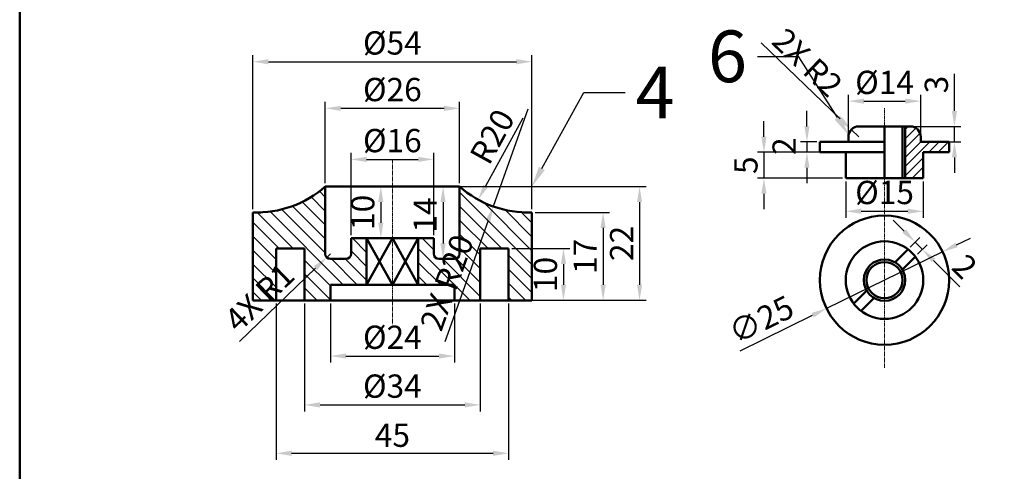
# Model space of a CAD drawing. Units: millimetres. Extents: x 418 to 773, y -46 to 294.
# Tile 4 of 7: x 418 to 609, y 77 to 164. Entities that reach past the tile are written whole.
import ezdxf
from ezdxf import colors
from ezdxf.entities.mleader import LeaderData, LeaderLine
from ezdxf.math import Vec2, Vec3

# ---------------------------------------------------------------- set-up
doc = ezdxf.new("R2010")
doc.units = ezdxf.units.MM
doc.header["$LTSCALE"] = 0.2
doc.linetypes.add('CENTER2', pattern=[28.575, 19.05, -3.175, 3.175, -3.175])
for name, color, linetype, lineweight in [('M-CNTR', 1, 'CENTER2', 18), ('M-DIMS', 2, 'Continuous', 25), ('M-HATC', 8, 'Continuous', 18), ('M-OUTL', 7, 'Continuous', 50), ('M-TEXT', 3, 'Continuous', 25), ('M-TTLB', 7, 'Continuous', 50)]:
    doc.layers.add(name, color=color, linetype=linetype, lineweight=lineweight)
doc.styles.get("Standard").update_dxf_attribs({"font": 'arial.ttf'})
doc.dimstyles.new('ISO-25', dxfattribs={"dimtxt": 4.5, "dimasz": 3, "dimexe": 1.25, "dimexo": 0.625, "dimtad": 1, "dimdec": 1, "dimtxsty": 'Standard', "dimcen": 2.5, "dimadec": 0, "dimazin": 0, "dimtfac": 1, "dimtdec": 1, "dimtmove": 0, "dimatfit": 3, "dimfxl": 1, "dimarcsym": 0})

# ---------------------------------------------------------------- blocks, each defined once
blk = doc.blocks.new('*D22')
at = {"layer": 'Defpoints', "color": 0, "ltscale": 0.2, "transparency": 16777216}
for p in [(517.09, 155.7), (463.09, 126.57), (517.09, 126.57)]:
    blk.add_point(p, dxfattribs=at)
at = {"layer": 'M-DIMS', "color": 0, "lineweight": -2, "ltscale": 0.2, "transparency": 16777216}
for p, q in [((463.09, 127.19), (463.09, 156.95)), ((517.09, 127.19), (517.09, 156.95)), ((466.09, 155.7), (514.09, 155.7))]:
    blk.add_line(p, q, dxfattribs=at)
at = {"layer": 'M-DIMS', "color": 0, "ltscale": 0.2, "transparency": 16777216}
for points in [[(466.09, 156.2), (466.09, 155.2), (463.09, 155.7)], [(514.09, 156.2), (514.09, 155.2), (517.09, 155.7)]]:
    blk.add_solid(points, dxfattribs=at)
at = {"layer": 'M-DIMS', "color": 0, "ltscale": 0.2, "transparency": 16777216, "insert": (490.09, 158.75), "char_height": 4.5, "attachment_point": 5}
blk.add_mtext('%%C54', dxfattribs=at)
blk = doc.blocks.new('*D23')
at = {"layer": 'Defpoints', "color": 0, "ltscale": 0.2, "transparency": 16777216}
for p in [(503.09, 146.69), (477.09, 131.57), (503.09, 131.57)]:
    blk.add_point(p, dxfattribs=at)
at = {"layer": 'M-DIMS', "color": 0, "lineweight": -2, "ltscale": 0.2, "transparency": 16777216}
for p, q in [((477.09, 132.19), (477.09, 147.94)), ((503.09, 132.19), (503.09, 147.94)), ((480.09, 146.69), (500.09, 146.69))]:
    blk.add_line(p, q, dxfattribs=at)
at = {"layer": 'M-DIMS', "color": 0, "ltscale": 0.2, "transparency": 16777216}
for points in [[(480.09, 147.19), (480.09, 146.19), (477.09, 146.69)], [(500.09, 147.19), (500.09, 146.19), (503.09, 146.69)]]:
    blk.add_solid(points, dxfattribs=at)
at = {"layer": 'M-DIMS', "color": 0, "ltscale": 0.2, "transparency": 16777216, "insert": (490.09, 149.74), "char_height": 4.5, "attachment_point": 5}
blk.add_mtext('%%C26', dxfattribs=at)
blk = doc.blocks.new('*D24')
at = {"layer": 'Defpoints', "color": 0, "ltscale": 0.2, "transparency": 16777216}
for p in [(497.65, 131.57), (502.09, 109.57), (537.94, 109.57)]:
    blk.add_point(p, dxfattribs=at)
at = {"layer": 'M-DIMS', "color": 0, "lineweight": -2, "ltscale": 0.2, "transparency": 16777216}
for p, q in [((498.28, 131.57), (539.19, 131.57)), ((537.94, 128.57), (537.94, 112.57)), ((502.72, 109.57), (539.19, 109.57))]:
    blk.add_line(p, q, dxfattribs=at)
at = {"layer": 'M-DIMS', "color": 0, "ltscale": 0.2, "transparency": 16777216}
for points in [[(537.44, 128.57), (538.44, 128.57), (537.94, 131.57)], [(537.44, 112.57), (538.44, 112.57), (537.94, 109.57)]]:
    blk.add_solid(points, dxfattribs=at)
at = {"layer": 'M-DIMS', "color": 0, "ltscale": 0.2, "transparency": 16777216, "insert": (535.05, 120.57), "char_height": 4.5, "attachment_point": 5, "rotation": 90}
blk.add_mtext('22', dxfattribs=at)
blk = doc.blocks.new('*D25')
at = {"layer": 'Defpoints', "color": 0, "ltscale": 0.2, "transparency": 16777216}
for p in [(517.09, 126.57), (517.09, 109.57), (530.88, 109.57)]:
    blk.add_point(p, dxfattribs=at)
at = {"layer": 'M-DIMS', "color": 0, "lineweight": -2, "ltscale": 0.2, "transparency": 16777216}
for p, q in [((517.72, 126.57), (532.13, 126.57)), ((530.88, 123.57), (530.88, 112.57)), ((517.72, 109.57), (532.13, 109.57))]:
    blk.add_line(p, q, dxfattribs=at)
at = {"layer": 'M-DIMS', "color": 0, "ltscale": 0.2, "transparency": 16777216}
for points in [[(530.38, 123.57), (531.38, 123.57), (530.88, 126.57)], [(530.38, 112.57), (531.38, 112.57), (530.88, 109.57)]]:
    blk.add_solid(points, dxfattribs=at)
at = {"layer": 'M-DIMS', "color": 0, "ltscale": 0.2, "transparency": 16777216, "insert": (528, 118.07), "char_height": 4.5, "attachment_point": 5, "rotation": 90}
blk.add_mtext('17', dxfattribs=at)
blk = doc.blocks.new('*D26')
at = {"layer": 'Defpoints', "color": 0, "ltscale": 0.2, "transparency": 16777216}
for p in [(512.59, 119.57), (512.59, 109.57), (523.21, 109.57)]:
    blk.add_point(p, dxfattribs=at)
at = {"layer": 'M-DIMS', "color": 0, "lineweight": -2, "ltscale": 0.2, "transparency": 16777216}
for p, q in [((513.22, 119.57), (524.46, 119.57)), ((523.21, 116.57), (523.21, 112.57)), ((513.22, 109.57), (524.46, 109.57))]:
    blk.add_line(p, q, dxfattribs=at)
at = {"layer": 'M-DIMS', "color": 0, "ltscale": 0.2, "transparency": 16777216}
for points in [[(522.71, 116.57), (523.71, 116.57), (523.21, 119.57)], [(522.71, 112.57), (523.71, 112.57), (523.21, 109.57)]]:
    blk.add_solid(points, dxfattribs=at)
at = {"layer": 'M-DIMS', "color": 0, "ltscale": 0.2, "transparency": 16777216, "insert": (520.29, 114.57), "char_height": 4.5, "attachment_point": 5, "rotation": 90}
blk.add_mtext('10', dxfattribs=at)
blk = doc.blocks.new('*D27')
at = {"layer": 'Defpoints', "color": 0, "ltscale": 0.2, "transparency": 16777216}
for p in [(478.09, 109.57), (502.09, 109.57), (502.09, 98.8)]:
    blk.add_point(p, dxfattribs=at)
at = {"layer": 'M-DIMS', "color": 0, "lineweight": -2, "ltscale": 0.2, "transparency": 16777216}
for p, q in [((478.09, 108.94), (478.09, 97.55)), ((502.09, 108.94), (502.09, 97.55)), ((481.09, 98.8), (499.09, 98.8))]:
    blk.add_line(p, q, dxfattribs=at)
at = {"layer": 'M-DIMS', "color": 0, "ltscale": 0.2, "transparency": 16777216}
for points in [[(481.09, 99.3), (481.09, 98.3), (478.09, 98.8)], [(499.09, 99.3), (499.09, 98.3), (502.09, 98.8)]]:
    blk.add_solid(points, dxfattribs=at)
at = {"layer": 'M-DIMS', "color": 0, "ltscale": 0.2, "transparency": 16777216, "insert": (490.09, 101.85), "char_height": 4.5, "attachment_point": 5}
blk.add_mtext('%%C24', dxfattribs=at)
blk = doc.blocks.new('*D28')
at = {"layer": 'Defpoints', "color": 0, "ltscale": 0.2, "transparency": 16777216}
for p in [(473.09, 109.57), (507.09, 109.57), (507.09, 89.35)]:
    blk.add_point(p, dxfattribs=at)
at = {"layer": 'M-DIMS', "color": 0, "lineweight": -2, "ltscale": 0.2, "transparency": 16777216}
for p, q in [((473.09, 108.94), (473.09, 88.1)), ((507.09, 108.94), (507.09, 88.1)), ((476.09, 89.35), (504.09, 89.35))]:
    blk.add_line(p, q, dxfattribs=at)
at = {"layer": 'M-DIMS', "color": 0, "ltscale": 0.2, "transparency": 16777216}
for points in [[(476.09, 89.85), (476.09, 88.85), (473.09, 89.35)], [(504.09, 89.85), (504.09, 88.85), (507.09, 89.35)]]:
    blk.add_solid(points, dxfattribs=at)
at = {"layer": 'M-DIMS', "color": 0, "ltscale": 0.2, "transparency": 16777216, "insert": (490.09, 92.4), "char_height": 4.5, "attachment_point": 5}
blk.add_mtext('%%C34', dxfattribs=at)
blk = doc.blocks.new('*D29')
at = {"layer": 'Defpoints', "color": 0, "ltscale": 0.2, "transparency": 16777216}
for p in [(467.59, 109.57), (512.59, 109.57), (512.59, 80)]:
    blk.add_point(p, dxfattribs=at)
at = {"layer": 'M-DIMS', "color": 0, "lineweight": -2, "ltscale": 0.2, "transparency": 16777216}
for p, q in [((467.59, 108.94), (467.59, 78.75)), ((512.59, 108.94), (512.59, 78.75)), ((470.59, 80), (509.59, 80))]:
    blk.add_line(p, q, dxfattribs=at)
at = {"layer": 'M-DIMS', "color": 0, "ltscale": 0.2, "transparency": 16777216}
for points in [[(470.59, 80.5), (470.59, 79.5), (467.59, 80)], [(509.59, 80.5), (509.59, 79.5), (512.59, 80)]]:
    blk.add_solid(points, dxfattribs=at)
at = {"layer": 'M-DIMS', "color": 0, "ltscale": 0.2, "transparency": 16777216, "insert": (490.09, 82.91), "char_height": 4.5, "attachment_point": 5}
blk.add_mtext('45', dxfattribs=at)
blk = doc.blocks.new('*D30')
at = {"layer": 'Defpoints', "color": 0, "ltscale": 0.2, "transparency": 16777216}
for p in [(516.34, 146.56), (506.69, 129.03)]:
    blk.add_point(p, dxfattribs=at)
at = {"layer": 'M-DIMS', "color": 0, "lineweight": -2, "ltscale": 0.2, "transparency": 16777216}
blk.add_line((515.37, 144.79), (508.14, 131.66), dxfattribs=at)
at = {"layer": 'M-DIMS', "color": 0, "ltscale": 0.2, "transparency": 16777216}
blk.add_solid([(507.7, 131.9), (508.58, 131.42), (506.69, 129.03)], dxfattribs=at)
at = {"layer": 'M-DIMS', "color": 0, "ltscale": 0.2, "transparency": 16777216, "insert": (509.92, 140.95), "char_height": 4.5, "attachment_point": 5, "rotation": 61.1742}
blk.add_mtext('R20', dxfattribs=at)
blk = doc.blocks.new('*D31')
at = {"layer": 'Defpoints', "color": 0, "ltscale": 0.2, "transparency": 16777216}
for p in [(498.09, 136.82), (482.09, 121.57), (498.09, 121.57)]:
    blk.add_point(p, dxfattribs=at)
at = {"layer": 'M-DIMS', "color": 0, "lineweight": -2, "ltscale": 0.2, "transparency": 16777216}
for p, q in [((482.09, 122.19), (482.09, 138.07)), ((498.09, 122.19), (498.09, 138.07)), ((485.09, 136.82), (495.09, 136.82))]:
    blk.add_line(p, q, dxfattribs=at)
at = {"layer": 'M-DIMS', "color": 0, "ltscale": 0.2, "transparency": 16777216}
for points in [[(485.09, 137.32), (485.09, 136.32), (482.09, 136.82)], [(495.09, 137.32), (495.09, 136.32), (498.09, 136.82)]]:
    blk.add_solid(points, dxfattribs=at)
at = {"layer": 'M-DIMS', "color": 0, "ltscale": 0.2, "transparency": 16777216, "insert": (490.09, 139.87), "char_height": 4.5, "attachment_point": 5}
blk.add_mtext('%%C16', dxfattribs=at)
blk = doc.blocks.new('*D32')
at = {"layer": 'Defpoints', "color": 0, "ltscale": 0.2, "transparency": 16777216}
for p in [(499.92, 131.57), (499.9, 117.57), (500.59, 117.57)]:
    blk.add_point(p, dxfattribs=at)
at = {"layer": 'M-DIMS', "color": 0, "lineweight": -2, "ltscale": 0.2, "transparency": 16777216}
for p, q in [((499.29, 131.57), (498.65, 131.57)), ((499.9, 128.57), (499.9, 120.57)), ((499.97, 117.57), (498.65, 117.57))]:
    blk.add_line(p, q, dxfattribs=at)
at = {"layer": 'M-DIMS', "color": 0, "ltscale": 0.2, "transparency": 16777216}
for points in [[(499.4, 128.57), (500.4, 128.57), (499.9, 131.57)], [(499.4, 120.57), (500.4, 120.57), (499.9, 117.57)]]:
    blk.add_solid(points, dxfattribs=at)
at = {"layer": 'M-DIMS', "color": 0, "ltscale": 0.2, "transparency": 16777216, "insert": (497.02, 126.06), "char_height": 4.5, "attachment_point": 5, "rotation": 90}
blk.add_mtext('14', dxfattribs=at)
blk = doc.blocks.new('*D33')
at = {"layer": 'Defpoints', "color": 0, "ltscale": 0.2, "transparency": 16777216}
for p in [(490.09, 131.57), (487.85, 121.57), (490.09, 121.57)]:
    blk.add_point(p, dxfattribs=at)
at = {"layer": 'M-DIMS', "color": 0, "lineweight": -2, "ltscale": 0.2, "transparency": 16777216}
for p, q in [((489.47, 131.57), (486.6, 131.57)), ((487.85, 128.57), (487.85, 124.57)), ((489.47, 121.57), (486.6, 121.57))]:
    blk.add_line(p, q, dxfattribs=at)
at = {"layer": 'M-DIMS', "color": 0, "ltscale": 0.2, "transparency": 16777216}
for points in [[(487.35, 128.57), (488.35, 128.57), (487.85, 131.57)], [(487.35, 124.57), (488.35, 124.57), (487.85, 121.57)]]:
    blk.add_solid(points, dxfattribs=at)
at = {"layer": 'M-DIMS', "color": 0, "ltscale": 0.2, "transparency": 16777216, "insert": (484.93, 126.57), "char_height": 4.5, "attachment_point": 5, "rotation": 90}
blk.add_mtext('10', dxfattribs=at)
blk = doc.blocks.new('*D34')
at = {"layer": 'Defpoints', "color": 0, "ltscale": 0.2, "transparency": 16777216}
for p in [(592.37, 148.08), (578.37, 141.19), (592.37, 141.19)]:
    blk.add_point(p, dxfattribs=at)
at = {"layer": 'M-DIMS', "color": 0, "lineweight": -2, "ltscale": 0.2, "transparency": 16777216}
for p, q in [((578.37, 141.81), (578.37, 149.33)), ((592.37, 141.81), (592.37, 149.33)), ((581.37, 148.08), (589.37, 148.08))]:
    blk.add_line(p, q, dxfattribs=at)
at = {"layer": 'M-DIMS', "color": 0, "ltscale": 0.2, "transparency": 16777216}
for points in [[(581.37, 148.58), (581.37, 147.58), (578.37, 148.08)], [(589.37, 148.58), (589.37, 147.58), (592.37, 148.08)]]:
    blk.add_solid(points, dxfattribs=at)
at = {"layer": 'M-DIMS', "color": 0, "ltscale": 0.2, "transparency": 16777216, "insert": (585.37, 151.12), "char_height": 4.5, "attachment_point": 5}
blk.add_mtext('%%C14', dxfattribs=at)
blk = doc.blocks.new('*D35')
at = {"layer": 'Defpoints', "color": 0, "ltscale": 0.2, "transparency": 16777216}
for p in [(572.87, 140.19), (570.35, 138.19), (572.87, 138.19)]:
    blk.add_point(p, dxfattribs=at)
at = {"layer": 'M-DIMS', "color": 0, "lineweight": -2, "ltscale": 0.2, "transparency": 16777216}
for p, q in [((570.35, 143.19), (570.35, 146.19)), ((572.24, 140.19), (569.1, 140.19)), ((570.35, 140.19), (570.35, 138.19)), ((572.24, 138.19), (569.1, 138.19)), ((570.35, 135.19), (570.35, 132.19))]:
    blk.add_line(p, q, dxfattribs=at)
at = {"layer": 'M-DIMS', "color": 0, "ltscale": 0.2, "transparency": 16777216}
for points in [[(569.85, 143.19), (570.85, 143.19), (570.35, 140.19)], [(569.85, 135.19), (570.85, 135.19), (570.35, 138.19)]]:
    blk.add_solid(points, dxfattribs=at)
at = {"layer": 'M-DIMS', "color": 0, "ltscale": 0.2, "transparency": 16777216, "insert": (566.51, 139.38), "char_height": 4.5, "attachment_point": 5, "rotation": 90}
blk.add_mtext('2', dxfattribs=at)
blk = doc.blocks.new('*D36')
at = {"layer": 'Defpoints', "color": 0, "ltscale": 0.2, "transparency": 16777216}
for p in [(577.87, 138.19), (562.02, 133.19), (577.87, 133.19)]:
    blk.add_point(p, dxfattribs=at)
at = {"layer": 'M-DIMS', "color": 0, "lineweight": -2, "ltscale": 0.2, "transparency": 16777216}
for p, q in [((562.02, 141.19), (562.02, 144.19)), ((577.24, 138.19), (560.77, 138.19)), ((562.02, 138.19), (562.02, 133.19)), ((577.24, 133.19), (560.77, 133.19)), ((562.02, 130.19), (562.02, 127.19))]:
    blk.add_line(p, q, dxfattribs=at)
at = {"layer": 'M-DIMS', "color": 0, "ltscale": 0.2, "transparency": 16777216}
for points in [[(561.52, 141.19), (562.52, 141.19), (562.02, 138.19)], [(561.52, 130.19), (562.52, 130.19), (562.02, 133.19)]]:
    blk.add_solid(points, dxfattribs=at)
at = {"layer": 'M-DIMS', "color": 0, "ltscale": 0.2, "transparency": 16777216, "insert": (559.11, 135.69), "char_height": 4.5, "attachment_point": 5, "rotation": 90}
blk.add_mtext('5', dxfattribs=at)
blk = doc.blocks.new('*D37')
at = {"layer": 'Defpoints', "color": 0, "ltscale": 0.2, "transparency": 16777216}
for p in [(590.37, 143.19), (595.12, 140.19), (598.9, 140.19)]:
    blk.add_point(p, dxfattribs=at)
at = {"layer": 'M-DIMS', "color": 0, "lineweight": -2, "ltscale": 0.2, "transparency": 16777216}
for p, q in [((598.9, 146.19), (598.9, 153.39)), ((590.99, 143.19), (600.15, 143.19)), ((598.9, 140.19), (598.9, 143.19)), ((595.74, 140.19), (600.15, 140.19)), ((598.9, 137.19), (598.9, 134.19))]:
    blk.add_line(p, q, dxfattribs=at)
at = {"layer": 'M-DIMS', "color": 0, "ltscale": 0.2, "transparency": 16777216}
for points in [[(598.4, 146.19), (599.4, 146.19), (598.9, 143.19)], [(598.4, 137.19), (599.4, 137.19), (598.9, 140.19)]]:
    blk.add_solid(points, dxfattribs=at)
at = {"layer": 'M-DIMS', "color": 0, "ltscale": 0.2, "transparency": 16777216, "insert": (595.98, 151.29), "char_height": 4.5, "attachment_point": 5, "rotation": 90}
blk.add_mtext('3', dxfattribs=at)
blk = doc.blocks.new('*D38')
at = {"layer": 'Defpoints', "color": 0, "ltscale": 0.2, "transparency": 16777216}
for p in [(577.87, 133.19), (592.87, 133.19), (592.87, 126.79)]:
    blk.add_point(p, dxfattribs=at)
at = {"layer": 'M-DIMS', "color": 0, "lineweight": -2, "ltscale": 0.2, "transparency": 16777216}
for p, q in [((577.87, 132.56), (577.87, 125.54)), ((592.87, 132.56), (592.87, 125.54)), ((580.87, 126.79), (589.87, 126.79))]:
    blk.add_line(p, q, dxfattribs=at)
at = {"layer": 'M-DIMS', "color": 0, "ltscale": 0.2, "transparency": 16777216}
for points in [[(580.87, 127.29), (580.87, 126.29), (577.87, 126.79)], [(589.87, 127.29), (589.87, 126.29), (592.87, 126.79)]]:
    blk.add_solid(points, dxfattribs=at)
at = {"layer": 'M-DIMS', "color": 0, "ltscale": 0.2, "transparency": 16777216, "insert": (585.37, 129.84), "char_height": 4.5, "attachment_point": 5}
blk.add_mtext('%%C15', dxfattribs=at)
blk = doc.blocks.new('*D39')
at = {"layer": 'Defpoints', "color": 0, "ltscale": 0.2, "transparency": 16777216}
for p in [(589.92, 119.44), (592.72, 119.41), (591.33, 118.03)]:
    blk.add_point(p, dxfattribs=at)
at = {"layer": 'M-DIMS', "color": 0, "lineweight": -2, "ltscale": 0.2, "transparency": 16777216}
for p, q in [((589.18, 122.95), (587.06, 125.07)), ((590.36, 119.88), (592.19, 121.71)), ((591.3, 120.83), (592.72, 119.41)), ((591.77, 118.47), (593.6, 120.3)), ((594.84, 117.29), (599.95, 112.18))]:
    blk.add_line(p, q, dxfattribs=at)
at = {"layer": 'M-DIMS', "color": 0, "ltscale": 0.2, "transparency": 16777216}
for points in [[(589.53, 123.3), (588.83, 122.6), (591.3, 120.83)], [(595.19, 117.65), (594.48, 116.94), (592.72, 119.41)]]:
    blk.add_solid(points, dxfattribs=at)
at = {"layer": 'M-DIMS', "color": 0, "ltscale": 0.2, "transparency": 16777216, "insert": (600.49, 115.71), "char_height": 4.5, "attachment_point": 5, "rotation": 315}
blk.add_mtext('2', dxfattribs=at)
blk = doc.blocks.new('*D40')
at = {"layer": 'Defpoints', "color": 0, "ltscale": 0.2, "transparency": 16777216}
for p in [(596.6, 118.96), (574.13, 107.99)]:
    blk.add_point(p, dxfattribs=at)
at = {"layer": 'M-DIMS', "color": 0, "lineweight": -2, "ltscale": 0.2, "transparency": 16777216}
for p, q in [((599.3, 120.28), (601.99, 121.6)), ((596.6, 118.96), (574.13, 107.99)), ((557.4, 99.82), (571.44, 106.68))]:
    blk.add_line(p, q, dxfattribs=at)
at = {"layer": 'M-DIMS', "color": 0, "ltscale": 0.2, "transparency": 16777216}
for points in [[(599.08, 120.73), (599.51, 119.83), (596.6, 118.96)], [(571.22, 107.13), (571.66, 106.23), (574.13, 107.99)]]:
    blk.add_solid(points, dxfattribs=at)
at = {"layer": 'M-DIMS', "color": 0, "ltscale": 0.2, "transparency": 16777216, "insert": (561.73, 105.33), "char_height": 4.5, "attachment_point": 5, "rotation": 26.0258}
blk.add_mtext('∅25', dxfattribs=at)
blk = doc.blocks.new('*D99')
at = {"layer": 'Defpoints', "color": 0, "ltscale": 0.2, "transparency": 16777216}
for p in [(516.34, 146.56), (509.61, 127.72)]:
    blk.add_point(p, dxfattribs=at)
at = {"layer": 'M-DIMS', "color": 0, "lineweight": -2, "ltscale": 0.2, "transparency": 16777216}
for p, q in [((516.34, 146.56), (509.61, 127.72)), ((500.28, 101.6), (508.6, 124.9))]:
    blk.add_line(p, q, dxfattribs=at)
at = {"layer": 'M-DIMS', "color": 0, "ltscale": 0.2, "transparency": 16777216}
blk.add_solid([(508.13, 125.06), (509.07, 124.73), (509.61, 127.72)], dxfattribs=at)
at = {"layer": 'M-DIMS', "color": 0, "ltscale": 0.2, "transparency": 16777216, "insert": (501.18, 112.82), "char_height": 4.5, "attachment_point": 5, "rotation": 70.3455}
blk.add_mtext('2X R20', dxfattribs=at)
blk = doc.blocks.new('*D100')
at = {"layer": 'Defpoints', "color": 0, "ltscale": 0.2, "transparency": 16777216}
for p in [(478.09, 118.57), (477.37, 117.88)]:
    blk.add_point(p, dxfattribs=at)
at = {"layer": 'M-DIMS', "color": 0, "lineweight": -2, "ltscale": 0.2, "transparency": 16777216}
for p, q in [((478.09, 118.57), (477.37, 117.88)), ((460.46, 101.58), (475.21, 115.79))]:
    blk.add_line(p, q, dxfattribs=at)
at = {"layer": 'M-DIMS', "color": 0, "ltscale": 0.2, "transparency": 16777216}
blk.add_solid([(474.86, 116.15), (475.56, 115.43), (477.37, 117.88)], dxfattribs=at)
at = {"layer": 'M-DIMS', "color": 0, "ltscale": 0.2, "transparency": 16777216, "insert": (464.75, 109.72), "char_height": 4.5, "attachment_point": 5, "rotation": 43.9304}
blk.add_mtext('4X R1', dxfattribs=at)
blk = doc.blocks.new('*D110')
at = {"layer": 'Defpoints', "color": 0, "ltscale": 0.2, "transparency": 16777216}
for p in [(578.93, 142.58), (580.37, 141.19)]:
    blk.add_point(p, dxfattribs=at)
at = {"layer": 'M-DIMS', "color": 0, "lineweight": -2, "ltscale": 0.2, "transparency": 16777216}
for p, q in [((561.48, 159.36), (576.76, 144.65)), ((580.37, 141.19), (578.93, 142.58))]:
    blk.add_line(p, q, dxfattribs=at)
at = {"layer": 'M-DIMS', "color": 0, "ltscale": 0.2, "transparency": 16777216}
blk.add_solid([(577.11, 145.02), (576.42, 144.29), (578.93, 142.58)], dxfattribs=at)
at = {"layer": 'M-DIMS', "color": 0, "ltscale": 0.2, "transparency": 16777216, "insert": (570.04, 155.13), "char_height": 4.5, "attachment_point": 5, "rotation": 316.11}
blk.add_mtext('2X R2', dxfattribs=at)

msp = doc.modelspace()

# ---------------------------------------------------------------- hatches: boundary and pattern name
at = {"layer": 'M-HATC', "ltscale": 0.2}
h = msp.add_hatch(dxfattribs=at)
h.set_pattern_fill('ANSI31', color=256, scale=0.4)
h.set_pattern_definition([(45, (-107.589, -89.179), (-0.8980256, 0.8980256), [])])
h.paths.add_polyline_path([(592.3673, 140.1885), (592.3673, 141.1885, 0.41421356), (590.3673, 143.1885), (589.3673, 143.1885), (589.3673, 133.1885), (592.8673, 133.1885), (592.8673, 138.1885), (597.8673, 138.1885), (597.8673, 140.1885)])
h = msp.add_hatch(dxfattribs=at)
h.set_pattern_fill('ANSI31', color=256, scale=0.6, angle=90)
h.set_pattern_definition([(135, (-147.1966, -57.104), (-1.3470384, -1.3470384), [])])
h.paths.add_polyline_path([(463.0912, 126.5696), (463.0912, 109.5696), (467.5912, 109.5696), (467.5912, 119.5696), (473.0912, 119.5696), (473.0912, 109.5696), (478.0912, 109.5696), (478.0912, 112.5696), (485.0912, 112.5696), (485.0912, 121.5696), (482.0912, 121.5696), (482.0912, 118.5696, -0.41421356), (481.0912, 117.5696), (478.0912, 117.5696, -0.41421356), (477.0912, 118.5696), (477.0912, 131.5696, -0.1927282)])
h.paths.add_polyline_path([(512.5912, 119.5696), (512.5912, 109.5696), (517.0912, 109.5696), (517.0912, 126.5696, -0.1927282), (503.0912, 131.5696), (503.0912, 118.5696, -0.41421356), (502.0912, 117.5696), (499.0912, 117.5696, -0.41421356), (498.0912, 118.5696), (498.0912, 121.5696), (495.0912, 121.5696), (495.0912, 112.5696), (502.0912, 112.5696), (502.0912, 109.5696), (507.0912, 109.5696), (507.0912, 119.5696)])

# ---------------------------------------------------------------- linework, layer by layer
at = {"layer": 'M-CNTR', "ltscale": 0.2}
for p, q in [((585.3673, 96.5498), (585.3673, 146.6995)), ((490.0912, 136.8195), (490.0912, 104.8482))]:
    msp.add_line(p, q, dxfattribs=at)
at = {"layer": 'M-OUTL', "ltscale": 0.2}
for p, q in [((590.3673, 143.1885), (580.3673, 143.1885)), ((585.3673, 143.1885), (585.3673, 133.1885)), ((588.8673, 143.1885), (588.8673, 133.1885)), ((589.3673, 143.1885), (589.3673, 133.1885)), ((578.3673, 141.1885), (578.3673, 140.1885)), ((592.3673, 140.1885), (592.3673, 141.1885)), ((572.8673, 140.1885), (572.8673, 138.2414)), ((585.3673, 140.1885), (572.8673, 140.1885)), ((597.8673, 140.1885), (592.3673, 140.1885)), ((597.8673, 138.1885), (597.8673, 140.1885)), ((572.8673, 138.2414), (572.8673, 138.1885)), ((572.8673, 138.1885), (585.3673, 138.1885)), ((577.8673, 138.1885), (577.8673, 133.1885)), ((592.8673, 133.1885), (592.8673, 138.1885)), ((592.8673, 138.1885), (597.8673, 138.1885)), ((503.0912, 131.5696), (477.0912, 131.5696)), ((477.0912, 131.5696), (477.0912, 118.5696)), ((503.0912, 131.5696), (503.0912, 118.5696)), ((577.8673, 133.1885), (585.3673, 133.1885)), ((585.3673, 133.1885), (592.8673, 133.1885)), ((463.0912, 126.5696), (463.0912, 109.5696)), ((464.6014, 126.5696), (463.0912, 126.5696)), ((517.0912, 126.5696), (515.581, 126.5696)), ((517.0912, 109.5696), (517.0912, 126.5696)), ((498.0912, 121.5696), (482.0912, 121.5696)), ((482.0912, 118.5696), (482.0912, 121.5696)), ((485.0912, 112.5696), (485.0912, 121.5696)), ((485.0912, 121.5696), (490.0912, 112.5696)), ((485.0912, 112.5696), (490.0912, 121.5696)), ((490.0912, 112.5696), (495.0912, 121.5696)), ((490.0912, 121.5696), (495.0912, 112.5696)), ((495.0912, 112.5696), (495.0912, 121.5696)), ((498.0912, 118.5696), (498.0912, 121.5696)), ((467.5912, 109.5696), (467.5912, 119.5696)), ((467.5912, 119.5696), (473.0912, 119.5696)), ((473.0912, 109.5696), (473.0912, 119.5696)), ((507.0912, 109.5696), (507.0912, 119.5696)), ((512.5912, 119.5696), (507.0912, 119.5696)), ((512.5912, 109.5696), (512.5912, 119.5696)), ((589.9162, 119.4416), (587.3988, 116.9242)), ((478.0912, 117.5696), (481.0912, 117.5696)), ((502.0912, 117.5696), (499.0912, 117.5696)), ((591.3304, 118.0273), (588.813, 115.51)), ((502.0912, 112.5696), (478.0912, 112.5696)), ((478.0912, 112.5696), (478.0912, 109.5696)), ((502.0912, 109.5696), (502.0912, 112.5696)), ((581.9216, 111.447), (579.4043, 108.9297)), ((463.0912, 109.5696), (517.0912, 109.5696)), ((583.3358, 110.0328), (580.8185, 107.5154))]:
    msp.add_line(p, q, dxfattribs=at)
for radius in [12.5, 7.5, 4, 3.5]:
    msp.add_circle((585.3673, 113.4785), radius, dxfattribs=at)
for centre, radius, start, end in [((580.3673, 141.1885), 2, 90, 180), ((590.3673, 141.1885), 2, 0, 90), ((463.8463, 146.5553), 20, 267.836305, 311.471343), ((516.3361, 146.5553), 20, 228.528657, 272.163695), ((478.0912, 118.5696), 1, 180, 270), ((481.0912, 118.5696), 1, 270, 0), ((499.0912, 118.5696), 1, 180, 270), ((502.0912, 118.5696), 1, 270, 0)]:
    msp.add_arc(centre, radius, start, end, dxfattribs=at)
at = {"layer": 'M-TTLB', "ltscale": 0.2}
msp.add_lwpolyline([(417.9371, 294.4119), (773.2687, 294.4119), (773.2687, -46.4726), (417.9371, -46.4726)], close=True, dxfattribs=at)

# ---------------------------------------------------------------- dimensions: what is measured, and where the dimension line sits
at = {"layer": 'M-DIMS', "ltscale": 0.2}
for center, mpoint, text, picture, middle in [((580.3673, 141.1885), (578.926, 142.575), '2X <>', '*D110', (570.0421, 155.1254)), ((516.3361, 146.5553), (509.6092, 127.7205), '2X <>', '*D99', (501.1838, 112.8196)), ((478.0912, 118.5696), (477.371, 117.8758), '4X <>', '*D100', (464.7506, 109.7249))]:
    dim = msp.add_radius_dim(center=center, mpoint=mpoint, text=text, dimstyle='ISO-25', override={"dimdec": 0, "dimlfac": 1, "dimrnd": 0, "dimzin": 0, "dimdsep": 46, "dimlunit": 2}, dxfattribs=at)
    dim.commit()
    dim.dimension.update_dxf_attribs({"geometry": picture, "text_midpoint": middle})
for base, p1, p2, picture, middle in [((517.0912, 155.6989), (463.0912, 126.5696), (517.0912, 126.5696), '*D22', (490.0912, 155.6989)), ((503.0912, 146.6915), (477.0912, 131.5696), (503.0912, 131.5696), '*D23', (490.0912, 146.6915)), ((498.0912, 136.8195), (482.0912, 121.5696), (498.0912, 121.5696), '*D31', (490.0912, 136.8195)), ((507.0912, 89.3545), (473.0912, 109.5696), (507.0912, 109.5696), '*D28', (490.0912, 89.3545)), ((502.0912, 98.8027), (478.0912, 109.5696), (502.0912, 109.5696), '*D27', (490.0912, 98.8027))]:
    dim = msp.add_linear_dim(base=base, p1=p1, p2=p2, text='%%C<>', dimstyle='ISO-25', override={"dimclrd": 0, "dimclre": 0, "dimclrt": 0}, dxfattribs=at)
    dim.commit()
    dim.dimension.update_dxf_attribs({"geometry": picture, "text_midpoint": middle, "dimtype": 160})
for base, p1, p2, picture, middle in [((592.3673, 148.0751), (578.3673, 141.1885), (592.3673, 141.1885), '*D34', (585.3673, 151.1236)), ((592.8673, 126.7868), (577.8673, 133.1885), (592.8673, 133.1885), '*D38', (585.3673, 129.8352))]:
    dim = msp.add_linear_dim(base=base, p1=p1, p2=p2, text='%%C<>', dimstyle='ISO-25', override={"dimclrd": 0, "dimclre": 0, "dimclrt": 0}, dxfattribs=at)
    dim.commit()
    dim.dimension.update_dxf_attribs({"geometry": picture, "text_midpoint": middle})
for base, p1, p2, override, picture, middle in [((598.902, 140.1885), (590.3673, 143.1885), (595.1173, 140.1885), {"dimclrd": 0, "dimclre": 0, "dimclrt": 0}, '*D37', (598.902, 151.2869)), ((570.3517, 138.1885), (572.8673, 140.1885), (572.8673, 138.1885), {"dimclrd": 0, "dimclre": 0, "dimclrt": 0, "dimtmove": 2}, '*D35', (566.5066, 139.3842)), ((499.902, 117.5696), (499.9157, 131.5696), (500.5912, 117.5696), {"dimclrd": 0, "dimclre": 0, "dimclrt": 0}, '*D32', (499.902, 126.0606)), ((523.21, 109.5696), (512.5912, 119.5696), (512.5912, 109.5696), {"dimclrd": 0, "dimclre": 0, "dimclrt": 0}, '*D26', (523.21, 114.5696))]:
    dim = msp.add_linear_dim(base=base, p1=p1, p2=p2, angle=90, dimstyle='ISO-25', override=override, dxfattribs=at)
    dim.commit()
    dim.dimension.update_dxf_attribs({"geometry": picture, "text_midpoint": middle, "dimtype": 160})
dim = msp.add_radius_dim(center=(516.3361, 146.5553), mpoint=(506.6932, 129.0335), dimstyle='ISO-25', override={"dimclrd": 0, "dimclre": 0, "dimclrt": 0}, dxfattribs=at)
dim.commit()
dim.dimension.update_dxf_attribs({"geometry": '*D30', "text_midpoint": (512.4759, 139.5411), "dimtype": 164})
for base, p1, p2, picture, middle in [((562.0229, 133.1885), (577.8673, 138.1885), (577.8673, 133.1885), '*D36', (559.1095, 135.6885)), ((487.8509, 121.5696), (490.0912, 131.5696), (490.0912, 121.5696), '*D33', (484.9283, 126.5696)), ((537.9358, 109.5696), (497.6526, 131.5696), (502.0912, 109.5696), '*D24', (535.0516, 120.5696)), ((530.8809, 109.5696), (517.0912, 126.5696), (517.0912, 109.5696), '*D25', (527.9967, 118.0696))]:
    dim = msp.add_linear_dim(base=base, p1=p1, p2=p2, angle=90, dimstyle='ISO-25', override={"dimclrd": 0, "dimclre": 0, "dimclrt": 0}, dxfattribs=at)
    dim.commit()
    dim.dimension.update_dxf_attribs({"geometry": picture, "text_midpoint": middle})
dim = msp.add_aligned_dim(p1=(589.9162, 119.4416), p2=(591.3304, 118.0273), distance=1.9604, dimstyle='ISO-25', override={"dimclrd": 0, "dimclre": 0, "dimclrt": 0}, dxfattribs=at)
dim.commit()
dim.dimension.update_dxf_attribs({"geometry": '*D39', "text_midpoint": (600.4944, 115.7147)})
dim = msp.add_diameter_dim_2p(p1=(596.5998, 118.9632), p2=(574.1349, 107.9938), dimstyle='ISO-25', override={"dimclrd": 0, "dimclre": 0, "dimclrt": 0}, dxfattribs=at)
dim.commit()
dim.dimension.update_dxf_attribs({"geometry": '*D40', "text_midpoint": (561.7329, 105.3305)})
dim = msp.add_linear_dim(base=(512.5912, 79.9985), p1=(467.5912, 109.5696), p2=(512.5912, 109.5696), dimstyle='ISO-25', override={"dimclrd": 0, "dimclre": 0, "dimclrt": 0}, dxfattribs=at)
dim.commit()
dim.dimension.update_dxf_attribs({"geometry": '*D29', "text_midpoint": (490.0912, 82.9119)})

# ---------------------------------------------------------------- leaders
at = {"layer": 'M-TEXT', "ltscale": 0.2}
ml = msp.add_multileader_mtext('Standard', dxfattribs=at)
ml.set_content('6', color=256)
ml.set_leader_properties()
ml.build(insert=Vec2(0, 0))
ctx = ml.context
ctx.base_point, ctx.char_height, ctx.plane_origin = Vec3(550.1461, 156.658), 10, Vec3(578.3955, 141.5228)
ctx.text_align_type = 2
notes = []
notes.append((ctx, [(0, (1, 1, 0), (568.7491, 156.658), (-1, 0), 8, [(0, [(578.3955, 141.5228)], 0, [])])]))
ctx.mtext.insert, ctx.mtext.alignment, ctx.mtext.flow_direction = Vec3(558.7491, 161.7432), 3, 5
ml = msp.add_multileader_mtext('Standard', dxfattribs=at)
ml.set_content('4', color=256)
ml.set_leader_properties()
ml.build(insert=Vec2(0, 0))
ctx = ml.context
ctx.base_point, ctx.char_height, ctx.plane_origin = Vec3(535.1623, 149.7591), 10, Vec3(517.0912, 131.5696)
notes.append((ctx, [(0, (1, 1, 0), (527.1623, 149.7591), (1, 0), 8, [(0, [(517.0912, 131.5696)], 0, [])])]))
ctx.mtext.insert, ctx.mtext.flow_direction = Vec3(537.1623, 154.7591), 5
for ctx, leaders in notes:
    for number, flags, end, landing, length, lines in leaders:
        leader = LeaderData()
        leader.index, (leader.has_last_leader_line, leader.has_dogleg_vector, leader.attachment_direction) = number, flags
        leader.last_leader_point, leader.dogleg_vector, leader.dogleg_length = Vec3(end), Vec3(landing), length
        for number, points, colour, breaks in lines:
            line = LeaderLine()
            line.index, line.vertices, line.color, line.breaks = number, Vec3.list(points), colors.encode_raw_color(colour), breaks
            leader.lines.append(line)
        ctx.leaders.append(leader)

doc.saveas('drawing.dxf')
